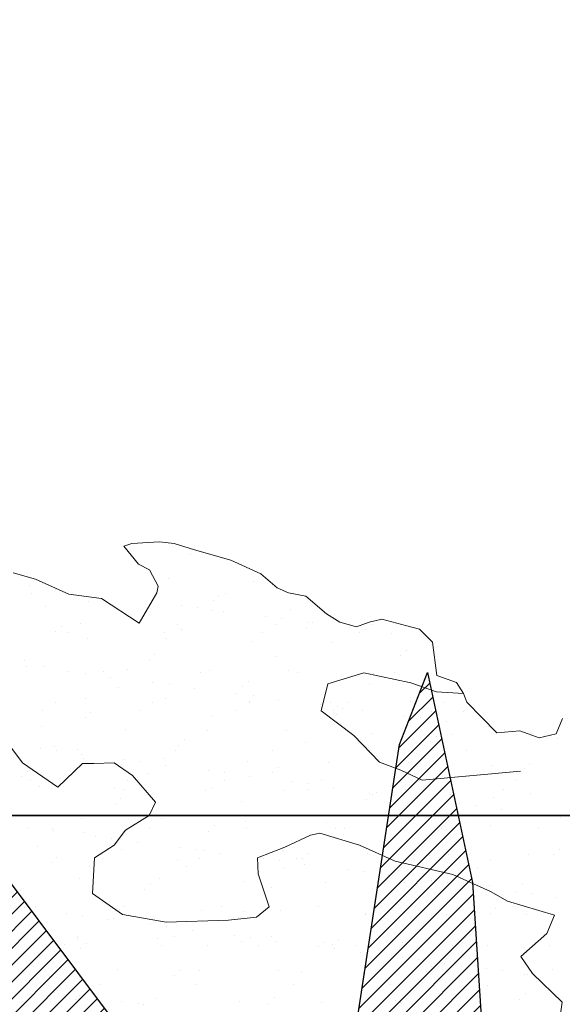
# Model space of a CAD drawing. Units: inches. Extents: x 1986 to 21484, y -1816 to 2016.
# Tile 37 of 85: x 2167.98 to 2174.94, y 1898.33 to 1910.95. Entities that reach past the tile are written whole.
import ezdxf

# ---------------------------------------------------------------- set-up
doc = ezdxf.new("R2010")
doc.units = ezdxf.units.IN
for name, color, linetype, lineweight in [('A-ANNO-DIMS', 2, 'Continuous', 18), ('C-PROP', 7, 'Continuous', 35), ('L-PLNT', 84, 'Continuous', 13), ('vfolhas', 114, 'Continuous', 5)]:
    doc.layers.add(name, color=color, linetype=linetype, lineweight=lineweight)
doc.layers.add('vfolha2', color=110, linetype='Continuous')
doc.layers.add('vfolhas2', color=102, linetype='Continuous')
doc.styles.get("Standard").update_dxf_attribs({"font": 'arial.ttf'})
doc.dimstyles.new('ISO-25', dxfattribs={"dimtxt": 8, "dimasz": 2.5, "dimexe": 1.25, "dimexo": 0.625, "dimtad": 1, "dimdec": 1, "dimlunit": 3, "dimtxsty": 'Standard', "dimcen": 2.5, "dimadec": 0, "dimazin": 0, "dimtfac": 1, "dimtdec": 1, "dimtmove": 0, "dimatfit": 3, "dimfxl": 1, "dimarcsym": 0})
pattern_1 = [(45, (-2446.5133113, 50.986076), (-0.004419417382, 0.004419417382), [])]

# ---------------------------------------------------------------- blocks, each defined once
blk = doc.blocks.new('*D1')
at = {"layer": 'A-ANNO-DIMS', "color": 0, "lineweight": -2, "transparency": 16777216}
for p, q in [((2042.312, 1901.377), (2042.312, 1914.655)), ((2402.312, 1901.377), (2402.312, 1914.655)), ((2044.812, 1913.405), (2399.812, 1913.405))]:
    blk.add_line(p, q, dxfattribs=at)
at = {"layer": 'A-ANNO-DIMS', "color": 0, "transparency": 16777216}
for points in [[(2044.812, 1913.821), (2044.812, 1912.988), (2042.312, 1913.405)], [(2399.812, 1913.821), (2399.812, 1912.988), (2402.312, 1913.405)]]:
    blk.add_solid(points, dxfattribs=at)
at = {"layer": 'Defpoints', "color": 0, "transparency": 16777216}
for p in [(2402.312, 1913.405), (2042.312, 1900.752), (2402.312, 1900.752)]:
    blk.add_point(p, dxfattribs=at)
at = {"layer": 'A-ANNO-DIMS', "color": 0, "transparency": 16777216, "insert": (2222.312, 1918.117), "char_height": 8, "attachment_point": 5}
blk.add_mtext("30'", dxfattribs=at)
blk = doc.blocks.new('arbusto_PB_verde_grande')
at = {"layer": 'vfolha2'}
h = blk.add_hatch(dxfattribs=at)
h.set_pattern_fill('ANSI31', color=256, scale=0.05, style=0)
h.set_pattern_definition(pattern_1)
h.paths.add_polyline_path([(0.02944, 0.35651), (0.00028, 0.09048), (0.02625, -0.03934), (0.047, 0.06233), (0.06189, 0.09731), (0.09372, 0.26573), (0.09955, 0.43473), (0.08789, 0.61313), (0.0645, 0.72266), (0.04988, 0.6851), (0.0236, 0.51294)])
h.paths.add_polyline_path([(0.30106, 0.43789), (0.14225, 0.24871), (0.26685, 0.30022)])
h.paths.add_polyline_path([(0.37995, 0.22817), (0.23697, 0.15193), (0.18428, 0.09364), (0.11122, 0.04358), (0.02625, -0.03934), (0.28061, 0.04667), (0.36829, 0.07798), (0.46756, 0.11239), (0.61068, 0.19376), (0.71585, 0.27823), (0.55813, 0.25948)])
h.paths.add_polyline_path([(0.56101, -0.29441), (0.72752, -0.32573), (0.59024, -0.2412), (0.42962, -0.15982), (0.02625, -0.03934), (0.14922, -0.14107), (0.18838, -0.16604), (0.41501, -0.24435)])
h.paths.add_polyline_path([(-0.27429, -0.44776), (-0.30352, -0.72628), (-0.23923, -0.64175), (-0.15457, -0.45716), (0.02625, -0.03934), (-0.16328, -0.25376)])
h.paths.add_polyline_path([(-0.51963, -0.24744), (-0.67736, -0.32573), (-0.59558, -0.35072), (-0.40574, -0.32882), (-0.21007, -0.20995), (0.02625, -0.03934), (-0.14874, -0.06595), (-0.31518, -0.09101), (-0.41452, -0.15048)])
h.paths.add_polyline_path([(-0.52546, 0.25007), (-0.70947, 0.24698), (-0.51963, 0.1093), (-0.32979, 0.02167), (-0.07567, -0.0128), (-0.04234, -0.02148), (-0.35024, 0.1312)])
at = {"layer": 'vfolhas'}
h = blk.add_hatch(dxfattribs=at)
h.set_pattern_fill('ANSI31', color=256, scale=0.05, style=0)
h.set_pattern_definition(pattern_1)
h.paths.add_polyline_path([(-0.07279, 0.50669), (-0.18085, 0.65063), (-0.2334, 0.67253), (-0.20712, 0.53176), (-0.10785, 0.25007), (0.02625, -0.03934), (0.00028, 0.09048), (0.00816, 0.16241), (-0.04939, 0.29079)])
h.paths.add_polyline_path([(0.09902, 0.41929), (0.09372, 0.26573), (0.07906, 0.18814), (0.15506, 0.36901), (0.26606, 0.5505), (0.28356, 0.63504), (0.2485, 0.68819), (0.25145, 0.63504), (0.20178, 0.54426)])
h.paths.add_polyline_path([(0.12295, 0.24073), (0.047, 0.06233), (0.02625, -0.03934), (0.11122, 0.04358), (0.18428, 0.09364), (0.27478, 0.19376), (0.3215, 0.25323), (0.44129, 0.38467), (0.47634, 0.57866), (0.41789, 0.45347), (0.28939, 0.30954)])
h.paths.add_polyline_path([(0.58145, -0.03779), (0.70707, 0.01536), (0.78591, 0.04667), (0.74796, 0.06549), (0.62818, 0.08423), (0.52595, 0.09048), (0.39745, 0.04358), (0.02625, -0.03934), (0.25728, -0.03154), (0.43834, -0.0347)])
h.paths.add_polyline_path([(0.52022, -0.03647), (0.43834, -0.0347), (0.25728, -0.03154), (0.02625, -0.03934), (0.17964, -0.08515), (0.53768, -0.13167), (0.69541, -0.15357), (0.78591, -0.07852), (0.70413, -0.10042)])
h.paths.add_polyline_path([(0.27189, -0.21929), (0.14922, -0.14107), (0.02625, -0.03934), (0.15794, -0.31007), (0.29522, -0.42585), (0.41789, -0.49157), (0.56396, -0.56669), (0.5114, -0.48532), (0.39456, -0.34139)])
h.paths.add_polyline_path([(-0.05818, -0.47591), (-0.02312, -0.61984), (0.047, -0.80134), (0.08494, -0.59794), (0.07911, -0.4071), (0.03527, -0.25376), (0.02625, -0.03934), (-0.03773, -0.26001)])
h.paths.add_polyline_path([(-0.24218, 0.14054), (-0.11073, 0.06858), (0.02625, -0.03934), (-0.04235, 0.10871), (-0.21007, 0.23757), (-0.36485, 0.33145), (-0.47874, 0.40341), (-0.54303, 0.46288), (-0.49041, 0.33145), (-0.39408, 0.22192)])
at = {"layer": 'vfolha2'}
for p, q in [((0.04988, 0.6851), (0.0645, 0.72266)), ((0.0645, 0.72266), (0.08789, 0.61313)), ((0.0236, 0.51294), (0.04988, 0.6851)), ((0.08789, 0.61313), (0.09955, 0.43473))]:
    blk.add_line(p, q, dxfattribs=at)
at = {"layer": 'vfolhas2'}
blk.add_line((-0.07279, 0.50669), (-0.18085, 0.65063), dxfattribs=at)
blk = doc.blocks.new('PLANT-SHRUB')
for p, q in [((2169.318, 1904.204), (2169.421, 1904.235)), ((2169.508, 1903.97), (2169.318, 1904.204)), ((2169.421, 1904.235), (2169.777, 1904.26)), ((2169.777, 1904.26), (2169.962, 1904.235)), ((2169.962, 1904.235), (2170.225, 1904.157)), ((2170.168, 1904.097), (2170.168, 1904.097)), ((2170.225, 1904.157), (2170.689, 1904.024)), ((2169.647, 1903.897), (2169.508, 1903.97)), ((2170.689, 1904.024), (2171.076, 1903.848)), ((2167.902, 1903.86), (2168.188, 1903.779)), ((2169.757, 1903.691), (2169.647, 1903.897)), ((2171.076, 1903.848), (2171.282, 1903.668)), ((2168.116, 1903.695), (2168.116, 1903.695)), ((2168.188, 1903.779), (2168.613, 1903.589)), ((2169.743, 1903.603), (2169.757, 1903.691)), ((2169.897, 1903.793), (2169.897, 1903.793)), ((2170.977, 1903.754), (2170.977, 1903.754)), ((2168.131, 1903.594), (2168.131, 1903.594)), ((2168.441, 1903.652), (2168.441, 1903.652)), ((2168.613, 1903.589), (2169.031, 1903.53)), ((2169.515, 1903.215), (2169.743, 1903.603)), ((2170.536, 1903.571), (2170.536, 1903.571)), ((2170.62, 1903.59), (2170.62, 1903.59)), ((2171.282, 1903.668), (2171.431, 1903.606)), ((2171.431, 1903.606), (2171.653, 1903.56)), ((2171.653, 1903.56), (2171.918, 1903.333)), ((2168.311, 1903.432), (2168.311, 1903.432)), ((2168.863, 1903.489), (2168.863, 1903.489)), ((2169.031, 1903.53), (2169.515, 1903.215)), ((2170.06, 1903.439), (2170.06, 1903.439)), ((2170.462, 1903.503), (2170.462, 1903.503)), ((2170.268, 1903.412), (2170.268, 1903.412)), ((2170.436, 1903.38), (2170.436, 1903.38)), ((2170.593, 1903.369), (2170.593, 1903.369)), ((2171.459, 1903.385), (2171.459, 1903.385)), ((2171.918, 1903.333), (2172.088, 1903.23)), ((2168.769, 1903.206), (2168.769, 1903.206)), ((2169.515, 1903.215), (2169.515, 1903.215)), ((2170.013, 1903.203), (2170.013, 1903.203)), ((2171.136, 1903.298), (2171.136, 1903.298)), ((2171.258, 1903.201), (2171.258, 1903.201)), ((2171.344, 1903.27), (2171.344, 1903.27)), ((2171.669, 1903.228), (2171.669, 1903.228)), ((2171.737, 1903.22), (2171.737, 1903.22)), ((2172.088, 1903.23), (2172.299, 1903.168)), ((2172.299, 1903.168), (2172.464, 1903.23)), ((2172.464, 1903.23), (2172.624, 1903.266)), ((2172.503, 1903.199), (2172.503, 1903.199)), ((2172.624, 1903.266), (2172.944, 1903.183)), ((2172.944, 1903.183), (2173.109, 1903.137)), ((2168.442, 1903.103), (2168.442, 1903.103)), ((2168.515, 1903.171), (2168.515, 1903.171)), ((2168.6, 1903.098), (2168.6, 1903.098)), ((2169.845, 1903.096), (2169.845, 1903.096)), ((2170.064, 1903.139), (2170.064, 1903.139)), ((2171.09, 1903.094), (2171.09, 1903.094)), ((2171.664, 1903.152), (2171.664, 1903.152)), ((2172.212, 1903.156), (2172.212, 1903.156)), ((2172.334, 1903.091), (2172.334, 1903.091)), ((2172.42, 1903.129), (2172.42, 1903.129)), ((2172.745, 1903.086), (2172.745, 1903.086)), ((2173.109, 1903.137), (2173.274, 1902.972)), ((2168.85, 1903.018), (2168.85, 1903.018)), ((2169.872, 1903.023), (2169.872, 1903.023)), ((2170.951, 1902.984), (2170.951, 1902.984)), ((2171.998, 1902.971), (2171.998, 1902.971)), ((2173.274, 1902.972), (2173.33, 1902.545)), ((2169.717, 1902.82), (2169.717, 1902.82)), ((2172.865, 1902.802), (2172.865, 1902.802)), ((2172.939, 1902.869), (2172.939, 1902.869)), ((2168.044, 1902.739), (2168.044, 1902.739)), ((2169.643, 1902.753), (2169.643, 1902.753)), ((2171.266, 1902.788), (2171.266, 1902.788)), ((2168.073, 1902.666), (2168.073, 1902.666)), ((2168.285, 1902.662), (2168.285, 1902.662)), ((2168.616, 1902.595), (2168.616, 1902.595)), ((2168.824, 1902.567), (2168.824, 1902.567)), ((2169.053, 1902.591), (2169.053, 1902.591)), ((2169.365, 1902.623), (2169.365, 1902.623)), ((2170.297, 1902.589), (2170.297, 1902.589)), ((2170.411, 1902.61), (2170.411, 1902.61)), ((2171.433, 1902.615), (2171.433, 1902.615)), ((2171.542, 1902.587), (2171.542, 1902.587)), ((2172.394, 1902.579), (2171.935, 1902.436)), ((2172.394, 1902.579), (2172.394, 1902.579)), ((2172.996, 1902.45), (2172.394, 1902.579)), ((2172.513, 1902.576), (2172.513, 1902.576)), ((2172.787, 1902.585), (2172.787, 1902.585)), ((2173.33, 1902.545), (2173.583, 1902.457)), ((2169.149, 1902.524), (2169.149, 1902.524)), ((2169.692, 1902.453), (2169.692, 1902.453)), ((2169.9, 1902.426), (2169.9, 1902.426)), ((2170.918, 1902.469), (2170.918, 1902.469)), ((2171.935, 1902.436), (2171.849, 1902.092)), ((2171.935, 1902.436), (2171.935, 1902.436)), ((2172.467, 1902.437), (2172.467, 1902.437)), ((2173.326, 1902.335), (2172.996, 1902.45)), ((2173.583, 1902.457), (2173.67, 1902.312)), ((2173.583, 1902.457), (2173.583, 1902.457)), ((2169.245, 1902.388), (2169.245, 1902.388)), ((2170.225, 1902.383), (2170.225, 1902.383)), ((2170.767, 1902.311), (2170.767, 1902.311)), ((2170.845, 1902.402), (2170.845, 1902.402)), ((2173.67, 1902.312), (2173.326, 1902.335)), ((2173.67, 1902.312), (2173.713, 1902.203)), ((2168.446, 1902.205), (2168.446, 1902.205)), ((2168.824, 1902.248), (2168.824, 1902.248)), ((2169.691, 1902.203), (2169.691, 1902.203)), ((2169.847, 1902.253), (2169.847, 1902.253)), ((2170.926, 1902.214), (2170.926, 1902.214)), ((2170.935, 1902.2), (2170.935, 1902.2)), ((2170.975, 1902.284), (2170.975, 1902.284)), ((2171.3, 1902.241), (2171.3, 1902.241)), ((2171.843, 1902.17), (2171.843, 1902.17)), ((2171.972, 1902.201), (2171.972, 1902.201)), ((2172.18, 1902.198), (2172.18, 1902.198)), ((2172.995, 1902.206), (2172.995, 1902.206)), ((2173.425, 1902.196), (2173.425, 1902.196)), ((2173.713, 1902.203), (2174.098, 1901.812)), ((2168.277, 1902.097), (2168.277, 1902.097)), ((2168.898, 1902.069), (2168.898, 1902.069)), ((2169.522, 1902.095), (2169.522, 1902.095)), ((2170.447, 1902.037), (2170.447, 1902.037)), ((2170.767, 1902.093), (2170.767, 1902.093)), ((2171.849, 1902.092), (2172.265, 1901.777)), ((2171.849, 1902.092), (2171.849, 1902.092)), ((2172.011, 1902.091), (2172.011, 1902.091)), ((2172.046, 1902.051), (2172.046, 1902.051)), ((2172.051, 1902.142), (2172.051, 1902.142)), ((2172.12, 1902.119), (2172.12, 1902.119)), ((2172.376, 1902.1), (2172.376, 1902.1)), ((2173.256, 1902.088), (2173.256, 1902.088)), ((2173.669, 1902.086), (2173.669, 1902.086)), ((2168.824, 1902.002), (2168.824, 1902.002)), ((2172.919, 1902.028), (2172.919, 1902.028)), ((2173.127, 1902.001), (2173.127, 1902.001)), ((2173.452, 1901.958), (2173.452, 1901.958)), ((2174.858, 1901.798), (2174.94, 1901.995)), ((2168.26, 1901.892), (2168.26, 1901.892)), ((2169.34, 1901.853), (2169.34, 1901.853)), ((2170.386, 1901.84), (2170.386, 1901.84)), ((2171.408, 1901.844), (2171.408, 1901.844)), ((2172.488, 1901.806), (2172.488, 1901.806)), ((2173.534, 1901.792), (2173.534, 1901.792)), ((2173.995, 1901.886), (2173.995, 1901.886)), ((2174.098, 1901.812), (2174.395, 1901.835)), ((2174.098, 1901.812), (2174.098, 1901.812)), ((2174.203, 1901.859), (2174.203, 1901.859)), ((2174.395, 1901.835), (2174.501, 1901.798)), ((2174.501, 1901.798), (2174.643, 1901.748)), ((2174.528, 1901.816), (2174.528, 1901.816)), ((2174.556, 1901.797), (2174.556, 1901.797)), ((2174.643, 1901.748), (2174.858, 1901.798)), ((2167.834, 1901.677), (2168.02, 1901.424)), ((2170.099, 1901.719), (2170.099, 1901.719)), ((2171.648, 1901.687), (2171.648, 1901.687)), ((2172.265, 1901.777), (2172.595, 1901.433)), ((2172.265, 1901.777), (2172.265, 1901.777)), ((2173.247, 1901.7), (2173.247, 1901.7)), ((2173.321, 1901.768), (2173.321, 1901.768)), ((2174.87, 1901.736), (2174.87, 1901.736)), ((2168.247, 1901.608), (2168.247, 1901.608)), ((2168.426, 1901.637), (2168.426, 1901.637)), ((2168.455, 1901.581), (2168.455, 1901.581)), ((2168.73, 1901.591), (2168.73, 1901.591)), ((2168.78, 1901.538), (2168.78, 1901.538)), ((2169.975, 1901.588), (2169.975, 1901.588)), ((2170.025, 1901.651), (2170.025, 1901.651)), ((2171.219, 1901.586), (2171.219, 1901.586)), ((2172.464, 1901.584), (2172.464, 1901.584)), ((2173.709, 1901.581), (2173.709, 1901.581)), ((2168.02, 1901.424), (2168.475, 1901.114)), ((2168.475, 1901.114), (2168.79, 1901.415)), ((2168.79, 1901.415), (2168.934, 1901.415)), ((2168.799, 1901.478), (2168.799, 1901.478)), ((2168.934, 1901.415), (2169.195, 1901.424)), ((2169.195, 1901.424), (2169.429, 1901.262)), ((2169.323, 1901.467), (2169.323, 1901.467)), ((2169.531, 1901.439), (2169.531, 1901.439)), ((2169.822, 1901.483), (2169.822, 1901.483)), ((2170.901, 1901.444), (2170.901, 1901.444)), ((2171.947, 1901.431), (2171.947, 1901.431)), ((2172.595, 1901.433), (2172.867, 1901.332)), ((2172.97, 1901.436), (2172.97, 1901.436)), ((2174.523, 1901.417), (2174.523, 1901.417)), ((2168.078, 1901.319), (2168.078, 1901.319)), ((2169.628, 1901.287), (2169.628, 1901.287)), ((2169.856, 1901.397), (2169.856, 1901.397)), ((2170.399, 1901.325), (2170.399, 1901.325)), ((2170.607, 1901.298), (2170.607, 1901.298)), ((2171.227, 1901.3), (2171.227, 1901.3)), ((2171.3, 1901.368), (2171.3, 1901.368)), ((2172.85, 1901.336), (2172.85, 1901.336)), ((2172.867, 1901.332), (2173.14, 1901.203)), ((2173.14, 1901.203), (2174.402, 1901.318)), ((2174.049, 1901.397), (2174.049, 1901.397)), ((2174.402, 1901.318), (2174.402, 1901.318)), ((2174.449, 1901.349), (2174.449, 1901.349)), ((2168.005, 1901.251), (2168.005, 1901.251)), ((2168.123, 1901.204), (2168.123, 1901.204)), ((2169.368, 1901.202), (2169.368, 1901.202)), ((2169.429, 1901.262), (2169.725, 1900.92)), ((2170.613, 1901.199), (2170.613, 1901.199)), ((2170.932, 1901.255), (2170.932, 1901.255)), ((2171.475, 1901.183), (2171.475, 1901.183)), ((2171.683, 1901.156), (2171.683, 1901.156)), ((2171.857, 1901.197), (2171.857, 1901.197)), ((2173.102, 1901.195), (2173.102, 1901.195)), ((2174.346, 1901.193), (2174.346, 1901.193)), ((2168.235, 1901.122), (2168.235, 1901.122)), ((2169.199, 1901.094), (2169.199, 1901.094)), ((2169.314, 1901.083), (2169.314, 1901.083)), ((2170.361, 1901.069), (2170.361, 1901.069)), ((2170.444, 1901.092), (2170.444, 1901.092)), ((2171.383, 1901.074), (2171.383, 1901.074)), ((2171.689, 1901.09), (2171.689, 1901.09)), ((2172.008, 1901.113), (2172.008, 1901.113)), ((2172.462, 1901.035), (2172.462, 1901.035)), ((2172.551, 1901.042), (2172.551, 1901.042)), ((2172.933, 1901.088), (2172.933, 1901.088)), ((2174.178, 1901.085), (2174.178, 1901.085)), ((2169.28, 1900.968), (2169.28, 1900.968)), ((2169.725, 1900.92), (2169.645, 1900.75)), ((2170.829, 1900.936), (2170.829, 1900.936)), ((2172.428, 1900.95), (2172.428, 1900.95)), ((2172.502, 1901.017), (2172.502, 1901.017)), ((2172.759, 1901.014), (2172.759, 1901.014)), ((2173.083, 1900.972), (2173.083, 1900.972)), ((2173.509, 1901.022), (2173.509, 1901.022)), ((2174.051, 1900.985), (2174.051, 1900.985)), ((2174.531, 1901.027), (2174.531, 1901.027)), ((2169.206, 1900.901), (2169.206, 1900.901)), ((2173.626, 1900.9), (2173.626, 1900.9)), ((2173.834, 1900.873), (2173.834, 1900.873)), ((2174.159, 1900.83), (2174.159, 1900.83)), ((2168.774, 1900.708), (2168.774, 1900.708)), ((2169.645, 1900.75), (2169.339, 1900.561)), ((2169.796, 1900.713), (2169.796, 1900.713)), ((2170.876, 1900.674), (2170.876, 1900.674)), ((2171.922, 1900.661), (2171.922, 1900.661)), ((2172.944, 1900.666), (2172.944, 1900.666)), ((2173.703, 1900.666), (2173.703, 1900.666)), ((2174.702, 1900.759), (2174.702, 1900.759)), ((2174.91, 1900.731), (2174.91, 1900.731)), ((2168.087, 1900.595), (2168.087, 1900.595)), ((2168.407, 1900.59), (2168.407, 1900.59)), ((2168.412, 1900.552), (2168.412, 1900.552)), ((2168.808, 1900.536), (2168.808, 1900.536)), ((2169.339, 1900.561), (2169.195, 1900.372)), ((2169.652, 1900.587), (2169.652, 1900.587)), ((2170.408, 1900.55), (2170.408, 1900.55)), ((2170.481, 1900.617), (2170.481, 1900.617)), ((2170.896, 1900.585), (2170.896, 1900.585)), ((2171.713, 1900.498), (2171.83, 1900.525)), ((2171.83, 1900.525), (2172.337, 1900.371)), ((2172.03, 1900.585), (2172.03, 1900.585)), ((2172.141, 1900.583), (2172.141, 1900.583)), ((2173.386, 1900.581), (2173.386, 1900.581)), ((2173.63, 1900.599), (2173.63, 1900.599)), ((2174.024, 1900.627), (2174.024, 1900.627)), ((2174.63, 1900.578), (2174.63, 1900.578)), ((2168.955, 1900.48), (2168.955, 1900.48)), ((2169.163, 1900.453), (2169.163, 1900.453)), ((2169.488, 1900.41), (2169.488, 1900.41)), ((2171.38, 1900.345), (2171.713, 1900.498)), ((2168.21, 1900.352), (2168.21, 1900.352)), ((2169.195, 1900.372), (2168.943, 1900.21)), ((2169.289, 1900.313), (2169.289, 1900.313)), ((2170.03, 1900.339), (2170.03, 1900.339)), ((2170.238, 1900.311), (2170.238, 1900.311)), ((2170.335, 1900.299), (2170.335, 1900.299)), ((2171.03, 1900.21), (2171.38, 1900.345)), ((2171.358, 1900.304), (2171.358, 1900.304)), ((2172.337, 1900.371), (2172.795, 1900.164)), ((2174.905, 1900.316), (2174.905, 1900.316)), ((2168.387, 1900.15), (2168.387, 1900.15)), ((2168.461, 1900.217), (2168.461, 1900.217)), ((2168.943, 1900.21), (2168.916, 1899.752)), ((2169.045, 1900.201), (2169.045, 1900.201)), ((2170.01, 1900.185), (2170.01, 1900.185)), ((2170.29, 1900.199), (2170.29, 1900.199)), ((2170.563, 1900.269), (2170.563, 1900.269)), ((2171.039, 1900.004), (2171.03, 1900.21)), ((2171.106, 1900.197), (2171.106, 1900.197)), ((2171.314, 1900.17), (2171.314, 1900.17)), ((2171.534, 1900.196), (2171.534, 1900.196)), ((2171.609, 1900.199), (2171.609, 1900.199)), ((2171.683, 1900.266), (2171.683, 1900.266)), ((2172.437, 1900.265), (2172.437, 1900.265)), ((2172.779, 1900.194), (2172.779, 1900.194)), ((2172.795, 1900.164), (2173.533, 1899.994)), ((2173.232, 1900.234), (2173.232, 1900.234)), ((2173.483, 1900.252), (2173.483, 1900.252)), ((2174.024, 1900.192), (2174.024, 1900.192)), ((2174.506, 1900.257), (2174.506, 1900.257)), ((2174.831, 1900.248), (2174.831, 1900.248)), ((2168.877, 1900.094), (2168.877, 1900.094)), ((2170.121, 1900.091), (2170.121, 1900.091)), ((2171.366, 1900.089), (2171.366, 1900.089)), ((2171.639, 1900.127), (2171.639, 1900.127)), ((2172.182, 1900.056), (2172.182, 1900.056)), ((2172.39, 1900.028), (2172.39, 1900.028)), ((2172.61, 1900.087), (2172.61, 1900.087)), ((2173.855, 1900.084), (2173.855, 1900.084)), ((2168.749, 1899.938), (2168.749, 1899.938)), ((2169.771, 1899.943), (2169.771, 1899.943)), ((2170.851, 1899.904), (2170.851, 1899.904)), ((2171.182, 1899.581), (2171.039, 1900.004)), ((2172.715, 1899.985), (2172.715, 1899.985)), ((2172.884, 1899.916), (2172.884, 1899.916)), ((2172.919, 1899.896), (2172.919, 1899.896)), ((2173.258, 1899.914), (2173.258, 1899.914)), ((2173.533, 1899.994), (2174.018, 1899.778)), ((2167.989, 1899.785), (2167.989, 1899.785)), ((2169.588, 1899.799), (2169.588, 1899.799)), ((2169.662, 1899.867), (2169.662, 1899.867)), ((2171.211, 1899.834), (2171.211, 1899.834)), ((2171.897, 1899.891), (2171.897, 1899.891)), ((2172.811, 1899.848), (2172.811, 1899.848)), ((2173.466, 1899.887), (2173.466, 1899.887)), ((2173.791, 1899.844), (2173.791, 1899.844)), ((2173.999, 1899.857), (2173.999, 1899.857)), ((2174.018, 1899.778), (2174.234, 1899.652)), ((2174.334, 1899.772), (2174.334, 1899.772)), ((2174.433, 1899.884), (2174.433, 1899.884)), ((2168.916, 1899.752), (2169.303, 1899.483)), ((2174.234, 1899.652), (2174.837, 1899.472)), ((2174.542, 1899.745), (2174.542, 1899.745)), ((2174.867, 1899.702), (2174.867, 1899.702)), ((2168.043, 1899.566), (2168.043, 1899.566)), ((2168.084, 1899.589), (2168.084, 1899.589)), ((2168.185, 1899.581), (2168.185, 1899.581)), ((2169.264, 1899.543), (2169.264, 1899.543)), ((2169.329, 1899.587), (2169.329, 1899.587)), ((2170.31, 1899.529), (2170.31, 1899.529)), ((2170.574, 1899.584), (2170.574, 1899.584)), ((2170.864, 1899.516), (2170.864, 1899.516)), ((2171.021, 1899.447), (2171.182, 1899.581)), ((2171.333, 1899.534), (2171.333, 1899.534)), ((2171.818, 1899.582), (2171.818, 1899.582)), ((2173.063, 1899.58), (2173.063, 1899.58)), ((2174.086, 1899.565), (2174.086, 1899.565)), ((2174.308, 1899.578), (2174.308, 1899.578)), ((2168.586, 1899.494), (2168.586, 1899.494)), ((2168.794, 1899.467), (2168.794, 1899.467)), ((2169.119, 1899.424), (2169.119, 1899.424)), ((2169.191, 1899.435), (2169.191, 1899.435)), ((2169.303, 1899.483), (2169.86, 1899.384)), ((2169.86, 1899.384), (2170.661, 1899.411)), ((2170.661, 1899.411), (2171.021, 1899.447)), ((2170.79, 1899.448), (2170.79, 1899.448)), ((2172.412, 1899.495), (2172.412, 1899.495)), ((2172.413, 1899.484), (2172.413, 1899.484)), ((2173.458, 1899.482), (2173.458, 1899.482)), ((2174.012, 1899.497), (2174.012, 1899.497)), ((2174.481, 1899.487), (2174.481, 1899.487)), ((2174.837, 1899.472), (2174.738, 1899.239)), ((2169.662, 1899.352), (2169.662, 1899.352)), ((2169.87, 1899.325), (2169.87, 1899.325)), ((2170.195, 1899.282), (2170.195, 1899.282)), ((2168.722, 1899.2), (2168.722, 1899.2)), ((2168.724, 1899.168), (2168.724, 1899.168)), ((2169.746, 1899.173), (2169.746, 1899.173)), ((2169.967, 1899.198), (2169.967, 1899.198)), ((2170.738, 1899.211), (2170.738, 1899.211)), ((2170.946, 1899.183), (2170.946, 1899.183)), ((2171.212, 1899.196), (2171.212, 1899.196)), ((2171.271, 1899.141), (2171.271, 1899.141)), ((2172.065, 1899.165), (2172.065, 1899.165)), ((2172.456, 1899.193), (2172.456, 1899.193)), ((2173.701, 1899.191), (2173.701, 1899.191)), ((2174.738, 1899.239), (2174.405, 1898.942)), ((2168.554, 1899.093), (2168.554, 1899.093)), ((2168.769, 1899.048), (2168.769, 1899.048)), ((2168.843, 1899.116), (2168.843, 1899.116)), ((2169.798, 1899.09), (2169.798, 1899.09)), ((2170.392, 1899.084), (2170.392, 1899.084)), ((2170.826, 1899.134), (2170.826, 1899.134)), ((2171.043, 1899.088), (2171.043, 1899.088)), ((2171.814, 1899.069), (2171.814, 1899.069)), ((2171.872, 1899.121), (2171.872, 1899.121)), ((2171.991, 1899.098), (2171.991, 1899.098)), ((2172.022, 1899.042), (2172.022, 1899.042)), ((2172.288, 1899.086), (2172.288, 1899.086)), ((2172.894, 1899.125), (2172.894, 1899.125)), ((2173.532, 1899.084), (2173.532, 1899.084)), ((2173.614, 1899.133), (2173.614, 1899.133)), ((2173.974, 1899.087), (2173.974, 1899.087)), ((2174.777, 1899.081), (2174.777, 1899.081)), ((2172.346, 1898.999), (2172.346, 1898.999)), ((2172.889, 1898.928), (2172.889, 1898.928)), ((2173.097, 1898.9), (2173.097, 1898.9)), ((2174.405, 1898.942), (2174.558, 1898.726)), ((2168.159, 1898.811), (2168.159, 1898.811)), ((2169.239, 1898.773), (2169.239, 1898.773)), ((2170.044, 1898.765), (2170.044, 1898.765)), ((2170.285, 1898.759), (2170.285, 1898.759)), ((2171.307, 1898.764), (2171.307, 1898.764)), ((2173.267, 1898.814), (2173.267, 1898.814)), ((2173.422, 1898.857), (2173.422, 1898.857)), ((2173.965, 1898.786), (2173.965, 1898.786)), ((2174.173, 1898.759), (2174.173, 1898.759)), ((2174.816, 1898.782), (2174.816, 1898.782)), ((2168.371, 1898.684), (2168.371, 1898.684)), ((2169.971, 1898.698), (2169.971, 1898.698)), ((2171.594, 1898.733), (2171.594, 1898.733)), ((2172.387, 1898.725), (2172.387, 1898.725)), ((2173.193, 1898.747), (2173.193, 1898.747)), ((2173.433, 1898.712), (2173.433, 1898.712)), ((2174.456, 1898.717), (2174.456, 1898.717)), ((2174.498, 1898.716), (2174.498, 1898.716)), ((2174.558, 1898.726), (2174.936, 1898.358)), ((2168.218, 1898.508), (2168.218, 1898.508)), ((2169.006, 1898.586), (2169.006, 1898.586)), ((2170.251, 1898.584), (2170.251, 1898.584)), ((2171.496, 1898.581), (2171.496, 1898.581)), ((2172.74, 1898.579), (2172.74, 1898.579)), ((2173.985, 1898.577), (2173.985, 1898.577)), ((2168.426, 1898.48), (2168.426, 1898.48)), ((2168.698, 1898.398), (2168.698, 1898.398)), ((2168.751, 1898.438), (2168.751, 1898.438)), ((2169.721, 1898.403), (2169.721, 1898.403)), ((2171.246, 1898.414), (2171.246, 1898.414)), ((2172.795, 1898.382), (2172.795, 1898.382)), ((2174.394, 1898.396), (2174.394, 1898.396)), ((2174.468, 1898.463), (2174.468, 1898.463)), ((2168.024, 1898.365), (2168.024, 1898.365)), ((2169.293, 1898.366), (2169.293, 1898.366)), ((2169.501, 1898.339), (2169.501, 1898.339)), ((2169.573, 1898.333), (2169.573, 1898.333)), ((2170.8, 1898.364), (2170.8, 1898.364)), ((2171.172, 1898.347), (2171.172, 1898.347)), ((2171.847, 1898.35), (2171.847, 1898.35)), ((2172.869, 1898.355), (2172.869, 1898.355)), ((2174.936, 1898.358), (2174.909, 1898.178))]:
    blk.add_line(p, q)

msp = doc.modelspace()

# ---------------------------------------------------------------- linework, layer by layer
at = {"layer": 'C-PROP'}
msp.add_lwpolyline([(2042.312, 1900.752), (2402.312, 1900.752), (2402.312, 1066.752), (2042.312, 1066.752)], close=True, dxfattribs=at)

# ---------------------------------------------------------------- block references
at = {"layer": 'L-PLNT'}
msp.add_blockref('PLANT-SHRUB', (0, 0), dxfattribs=at)
at = {"layer": 'L-PLNT', "xscale": 24.60366729364114, "yscale": 24.60366729364114, "zscale": 24.60366729364114}
msp.add_blockref('arbusto_PB_verde_grande', (2171.623, 1884.805), dxfattribs=at)

# ---------------------------------------------------------------- dimensions: what is measured, and where the dimension line sits
at = {"layer": 'A-ANNO-DIMS'}
dim = msp.add_linear_dim(base=(2402.312, 1913.405), p1=(2042.312, 1900.752), p2=(2402.312, 1900.752), dimstyle='ISO-25', override={"dimclrd": 0, "dimclre": 0, "dimclrt": 0}, dxfattribs=at)
dim.commit()
dim.dimension.update_dxf_attribs({"geometry": '*D1', "text_midpoint": (2222.312, 1918.117)})

doc.saveas('drawing.dxf')
